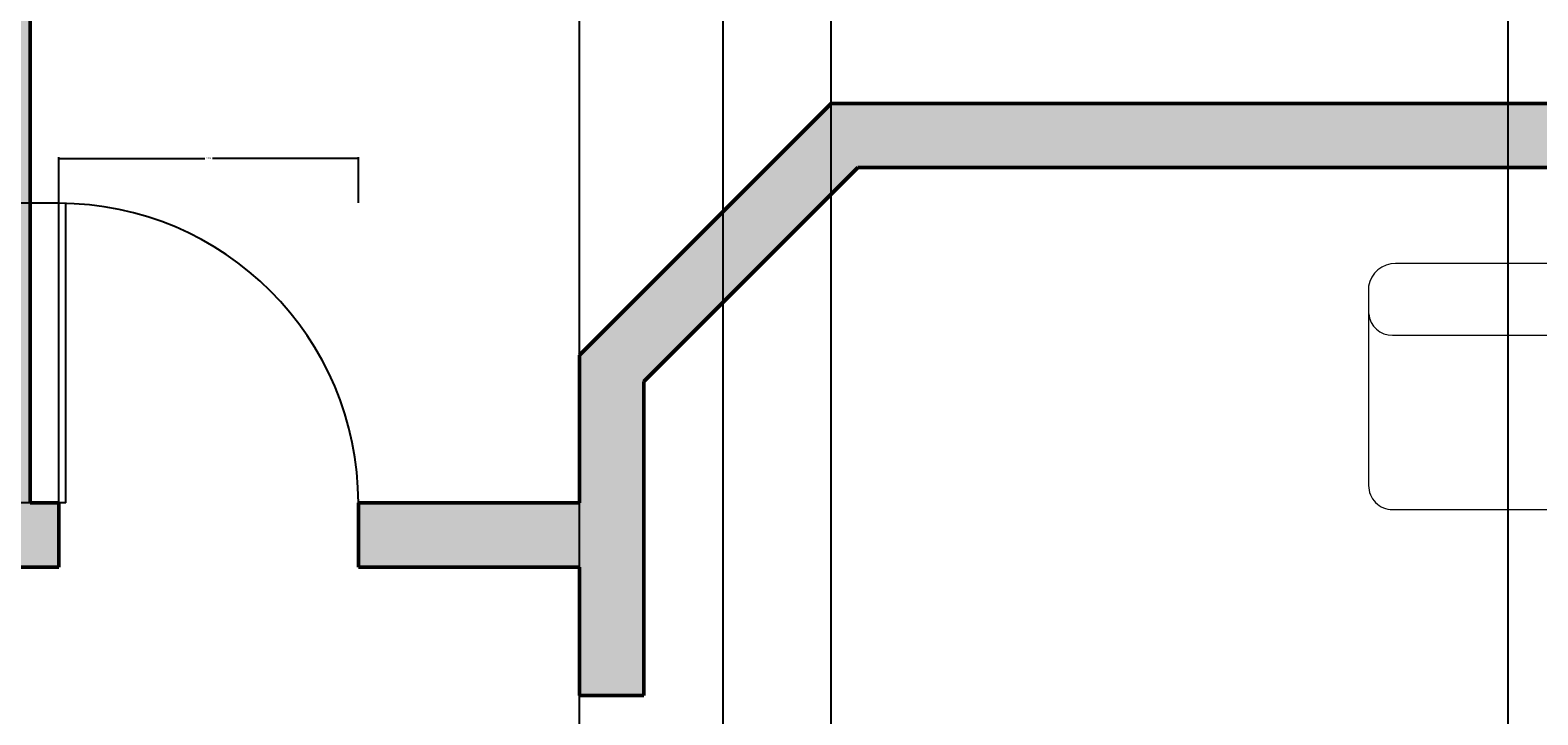
# Model space of a CAD drawing. Units: inches. Extents: x 2447 to 3157, y 2799 to 3988.
# Tile 4 of 9: x 2735 to 2947, y 3345 to 3441. Entities that reach past the tile are written whole.
import ezdxf

# ---------------------------------------------------------------- set-up
doc = ezdxf.new("R2010")
doc.units = ezdxf.units.IN
for name, color, linetype, lineweight in [('A-ANNO-DIMS', 2, 'Continuous', 18), ('A-DOOR', 3, 'Continuous', 25), ('A-FURN', 8, 'Continuous', 18), ('A-WALL', 7, 'Continuous', 50), ('A-WALL-PATT', 252, 'Continuous', 13)]:
    doc.layers.add(name, color=color, linetype=linetype, lineweight=lineweight)
doc.styles.get("Standard").update_dxf_attribs({"font": 'arial.ttf'})
doc.dimstyles.get("Standard").update_dxf_attribs({"dimtxt": 0.18, "dimasz": 0.18, "dimexe": 0.18, "dimexo": 0.0625, "dimgap": 0.09, "dimtad": 0, "dimtih": 1, "dimtoh": 1, "dimdec": 4, "dimzin": 0, "dimdsep": 46, "dimtxsty": 'Standard', "dimcen": 0.09, "dimadec": 0, "dimazin": 0, "dimtfac": 1, "dimtdec": 4, "dimtofl": 0, "dimtmove": 0, "dimatfit": 3, "dimfxl": 1, "dimtolj": 1, "dimtzin": 0, "dimarcsym": 0})

# ---------------------------------------------------------------- blocks, each defined once
blk = doc.blocks.new('A$C2F471D6A')
for p, q in [((2695.9, 2657.3), (2692.2, 1939.9)), ((1797.2, 841.3), (2182.6, 1242.6)), ((1797.2, 833.9), (2189.8, 1242.6)), ((1797.2, 826.4), (2197, 1242.6)), ((1797.2, 818.9), (2204.2, 1242.6)), ((1797.2, 848.8), (2175.4, 1242.6)), ((2161.4, 709.9), (2615.3, 1243.3)), ((2168.6, 709.9), (2622.5, 1243.3)), ((2175.8, 709.9), (2629.7, 1243.3)), ((2183, 709.9), (2636.9, 1243.3)), ((2190.2, 709.9), (2644.1, 1243.3)), ((2197.4, 709.9), (2651.3, 1243.3)), ((2755.3, 709.9), (2980.5, 1000.5)), ((2762.5, 709.9), (2981.1, 992)), ((2769.7, 709.9), (2981.1, 982.7)), ((2776.9, 709.9), (2981.1, 973.4)), ((2784.1, 709.9), (2981.1, 964.1)), ((807.3, 817.6), (89.9, 821.3))]:
    blk.add_line(p, q)
for points in [[(0, 1730, -0.393715), (947.4, 2744.8)], [(946.9, 2744.9, -1), (937.9, 2487, 1)], [(1060.8, 1939.9, 0.132391), (1145.9, 1873.4), (1778.5, 1873.4, 0.326313), (1874.7, 1943.6), (1874.7, 2657.3, 0.389129), (1793.3, 2746), (1149.6, 2746, 0.426582), (1064.5, 2657.3, 0.287811)], [(1060.8, 2545.7, 0.132391), (1145.9, 2479.2), (1778.5, 2479.2, 0.287096), (1869.3, 2536)], [(1878.2, 2536, 0.331063), (1959.6, 2475.5), (2433.2, 2475.5)], [(2433.2, 2475.5), (2592.3, 2475.5, 0.316456), (2692.2, 2545.7, 0.132391), (2777.2, 2479.2), (3409.9, 2479.2, 0.287096), (3500.7, 2536)], [(252.5, 1720.4), (252.5, 1729.1, -0.399385), (979.3, 2493.9)], [(812.9, 1633.4, 0.469502), (1063.7, 1935.5, -1.204519)], [(252.5, 1720.4, -0.77294), (0, 1730, -1)], [(257.4, 558.6), (257.4, 717.7, 0.316456), (187.2, 817.6, 0.132391), (253.7, 902.7), (253.7, 1535.3, 0.326313), (183.5, 1631.5), (180.9, 1631.5, 0.389129)], [(180.9, 0.4, 0.385191), (257.4, 85.1), (257.4, 558.6)]]:
    blk.add_lwpolyline(points, format="xyb")
for points in [[(2433.2, 1869.7), (2592.3, 1869.7, 0.316456), (2692.2, 1939.9, 0.132391), (2777.2, 1873.4), (3409.9, 1873.4, 0.326313), (3506.1, 1943.6), (3506.1, 2657.3, 0.389129), (3424.7, 2746), (2780.9, 2746, 0.426582), (2695.9, 2657.3, 0.287811), (2596, 2746), (1970.7, 2746, 0.366167), (1874.5, 2664.7), (1874.5, 1954.7, 0.414362), (1959.6, 1869.7)], [(877.5, 558.6), (877.5, 717.7, 0.316456), (807.3, 817.6, 0.132391), (873.8, 902.7), (873.8, 1535.3, 0.326313), (803.6, 1631.5), (89.9, 1631.5, 0.389129), (1.2, 1550.1), (1.2, 906.4, 0.426582), (89.9, 821.3, 0.287811), (1.2, 721.4), (1.2, 96.2, 0.366167), (82.5, 0), (792.5, 0, 0.414362), (877.5, 85.1)]]:
    blk.add_lwpolyline(points, format="xyb", close=True)
blk.add_lwpolyline([(1064.5, 2657.3), (1060.8, 1939.9)])
for points in [[(1742.1, 652.3), (1742.1, 1300.3), (3038.1, 1300.3), (3038.1, 652.3)], [(2981.1, 1185.5), (2920, 1185.5), (2920, 1242.6), (1860.2, 1242.6), (1860.2, 1185.5), (1797.2, 1185.5), (1797.2, 762.2), (1860.2, 762.2), (1860.2, 709.1), (2920, 709.1), (2920, 762.2), (2981.1, 762.2)]]:
    blk.add_lwpolyline(points, close=True)
blk = doc.blocks.new('DOOR-SWING-42IN')
for p, q in [((0, 0), (0, 42)), ((1, 0), (1, 41.99)), ((1, 0), (0, 0))]:
    blk.add_line(p, q)
blk.add_arc((0, 0), 42, 0, 90)
blk = doc.blocks.new('*D20')
at = {"layer": 'A-ANNO-DIMS', "color": 0, "lineweight": -2, "transparency": 16777216}
for p, q in [((2739.3, 3416.7), (2732.89, 3416.7)), ((2733.07, 3416.52), (2733.07, 3395.88)), ((2733.07, 3374.88), (2733.07, 3395.52)), ((2739.3, 3374.7), (2732.89, 3374.7))]:
    blk.add_line(p, q, dxfattribs=at)
at = {"layer": 'A-ANNO-DIMS', "color": 0, "transparency": 16777216}
for points in [[(2733.04, 3416.52), (2733.1, 3416.52), (2733.07, 3416.7)], [(2733.04, 3374.88), (2733.1, 3374.88), (2733.07, 3374.7)]]:
    blk.add_solid(points, dxfattribs=at)
at = {"layer": 'Defpoints', "color": 0, "transparency": 16777216}
for p in [(2733.07, 3416.7), (2739.37, 3416.7), (2739.37, 3374.7)]:
    blk.add_point(p, dxfattribs=at)
at = {"layer": 'A-ANNO-DIMS', "color": 0, "transparency": 16777216, "insert": (2733.07, 3395.7), "char_height": 0.18, "attachment_point": 5}
blk.add_mtext('\\A1;DOOR 42 TYP.', dxfattribs=at)
blk = doc.blocks.new('*D21')
at = {"layer": 'A-ANNO-DIMS', "color": 0, "lineweight": -2, "transparency": 16777216}
for p, q in [((2739.37, 3416.76), (2739.37, 3423.18)), ((2781.37, 3416.76), (2781.37, 3423.18)), ((2739.55, 3423), (2759.84, 3423)), ((2781.19, 3423), (2760.9, 3423))]:
    blk.add_line(p, q, dxfattribs=at)
at = {"layer": 'A-ANNO-DIMS', "color": 0, "transparency": 16777216}
for points in [[(2739.55, 3423.03), (2739.55, 3422.97), (2739.37, 3423)], [(2781.19, 3423.03), (2781.19, 3422.97), (2781.37, 3423)]]:
    blk.add_solid(points, dxfattribs=at)
at = {"layer": 'Defpoints', "color": 0, "transparency": 16777216}
for p in [(2781.37, 3423), (2739.37, 3416.7), (2781.37, 3416.7)]:
    blk.add_point(p, dxfattribs=at)
at = {"layer": 'A-ANNO-DIMS', "color": 0, "transparency": 16777216, "insert": (2760.37, 3423), "char_height": 0.18, "attachment_point": 5}
blk.add_mtext('\\A1;42 TYP.', dxfattribs=at)
blk = doc.blocks.new('*D47')
at = {"layer": 'A-ANNO-DIMS', "color": 0, "lineweight": -2, "transparency": 16777216}
for p, q in [((2798.43, 3849.7), (3156.7, 3849.7)), ((3156.52, 3849.52), (3156.52, 3487.38)), ((3156.52, 3124.88), (3156.52, 3487.02)), ((3046.43, 3124.7), (3156.7, 3124.7))]:
    blk.add_line(p, q, dxfattribs=at)
at = {"layer": 'A-ANNO-DIMS', "color": 0, "transparency": 16777216}
for points in [[(3156.49, 3849.52), (3156.55, 3849.52), (3156.52, 3849.7)], [(3156.49, 3124.88), (3156.55, 3124.88), (3156.52, 3124.7)]]:
    blk.add_solid(points, dxfattribs=at)
at = {"layer": 'Defpoints', "color": 0, "transparency": 16777216}
for p in [(2798.37, 3849.7), (3156.52, 3849.7), (3046.37, 3124.7)]:
    blk.add_point(p, dxfattribs=at)
at = {"layer": 'A-ANNO-DIMS', "color": 0, "transparency": 16777216, "insert": (3156.52, 3487.2), "char_height": 0.18, "attachment_point": 5}
blk.add_mtext('\\A1;725', dxfattribs=at)
blk = doc.blocks.new('*D50')
at = {"layer": 'A-ANNO-DIMS', "color": 0, "lineweight": -2, "transparency": 16777216}
for p, q in [((2832.46, 3897.64), (2832.46, 2799.37)), ((2942.46, 3897.64), (2942.46, 2799.37)), ((2832.64, 2799.55), (2887.18, 2799.55)), ((2942.28, 2799.55), (2887.74, 2799.55))]:
    blk.add_line(p, q, dxfattribs=at)
at = {"layer": 'A-ANNO-DIMS', "color": 0, "transparency": 16777216}
for points in [[(2832.64, 2799.58), (2832.64, 2799.52), (2832.46, 2799.55)], [(2942.28, 2799.58), (2942.28, 2799.52), (2942.46, 2799.55)]]:
    blk.add_solid(points, dxfattribs=at)
at = {"layer": 'Defpoints', "color": 0, "transparency": 16777216}
for p in [(2832.46, 3897.7), (2942.46, 3897.7), (2942.46, 2799.55)]:
    blk.add_point(p, dxfattribs=at)
at = {"layer": 'A-ANNO-DIMS', "color": 0, "transparency": 16777216, "insert": (2887.46, 2799.55), "char_height": 0.18, "attachment_point": 5}
blk.add_mtext('\\A1;110', dxfattribs=at)
blk = doc.blocks.new('*D73')
at = {"layer": 'A-ANNO-DIMS', "color": 0, "lineweight": -2, "transparency": 16777216}
for p, q in [((2812.37, 3160.03), (2812.37, 3988.03)), ((2812.55, 3987.85), (2829.61, 3987.85)), ((2847.46, 3987.85), (2830.4, 3987.85)), ((2847.64, 3124.76), (2847.64, 3988.03))]:
    blk.add_line(p, q, dxfattribs=at)
at = {"layer": 'A-ANNO-DIMS', "color": 0, "transparency": 16777216}
for points in [[(2812.55, 3987.88), (2812.55, 3987.82), (2812.37, 3987.85)], [(2847.46, 3987.88), (2847.46, 3987.82), (2847.64, 3987.85)]]:
    blk.add_solid(points, dxfattribs=at)
at = {"layer": 'Defpoints', "color": 0, "transparency": 16777216}
for p in [(2847.64, 3987.85), (2812.37, 3159.97), (2847.64, 3124.7)]:
    blk.add_point(p, dxfattribs=at)
at = {"layer": 'A-ANNO-DIMS', "color": 0, "transparency": 16777216, "insert": (2830, 3987.85), "char_height": 0.18, "attachment_point": 5}
blk.add_mtext('\\A1;35.27', dxfattribs=at)
blk = doc.blocks.new('*D76')
at = {"layer": 'A-ANNO-DIMS', "color": 0, "lineweight": -2, "transparency": 16777216}
for p, q in [((2847.64, 3124.76), (2847.64, 3988.03)), ((2847.82, 3987.85), (2908.95, 3987.85)), ((2970.99, 3987.85), (2909.86, 3987.85)), ((2971.17, 3124.76), (2971.17, 3988.03))]:
    blk.add_line(p, q, dxfattribs=at)
at = {"layer": 'A-ANNO-DIMS', "color": 0, "transparency": 16777216}
for points in [[(2847.82, 3987.88), (2847.82, 3987.82), (2847.64, 3987.85)], [(2970.99, 3987.88), (2970.99, 3987.82), (2971.17, 3987.85)]]:
    blk.add_solid(points, dxfattribs=at)
at = {"layer": 'Defpoints', "color": 0, "transparency": 16777216}
for p in [(2971.17, 3987.85), (2847.64, 3124.7), (2971.17, 3124.7)]:
    blk.add_point(p, dxfattribs=at)
at = {"layer": 'A-ANNO-DIMS', "color": 0, "transparency": 16777216, "insert": (2909.4, 3987.85), "char_height": 0.18, "attachment_point": 5}
blk.add_mtext('\\A1;123.53', dxfattribs=at)

msp = doc.modelspace()

# ---------------------------------------------------------------- hatches: boundary and pattern name
at = {"layer": 'A-WALL-PATT'}
h = msp.add_hatch(color=256, dxfattribs=at)
h.dxf.hatch_style = 1
h.paths.add_polyline_path([(2570.3672, 3550.7002), (2726.3672, 3550.7002), (2726.3672, 3370.7002), (2722.3672, 3370.7002), (2722.3672, 3365.7002), (2739.3672, 3365.7002), (2739.3672, 3374.7002), (2735.3672, 3374.7002), (2735.3672, 3563.7002), (2726.3672, 3563.7002), (2726.3672, 3559.7002), (2570.3672, 3559.7002), (2570.3672, 3599.2479), (2561.3672, 3599.2479), (2561.3672, 3508.7002), (2570.3672, 3508.7002)])
h.paths.add_polyline_path([(2570.3672, 3412.7002), (2561.3672, 3412.7002), (2561.3672, 3331.9279), (2570.3672, 3331.9279), (2570.3672, 3365.7002), (2666.3672, 3365.7002), (2666.3672, 3361.7002), (2671.3672, 3361.7002), (2671.3672, 3365.7002), (2686.3672, 3365.7002), (2686.3672, 3370.7002), (2570.3672, 3370.7002)])
h.paths.add_polyline_path([(2965.3672, 3430.7002), (2961.3672, 3430.7002), (2961.3672, 3434.7002), (2952.3672, 3434.7002), (2952.3672, 3430.7002), (2847.6393, 3430.7002), (2812.3672, 3395.4282), (2812.3672, 3374.7002), (2781.3672, 3374.7002), (2781.3672, 3365.7002), (2812.3672, 3365.7002), (2812.3672, 3347.7002), (2821.3672, 3347.7002), (2821.3672, 3391.7002), (2851.3672, 3421.7002), (2965.3672, 3421.7002)])
h.paths.add_polyline_path([(3046.3672, 3430.7002), (3033.3672, 3430.7002), (3033.3672, 3421.7002), (3037.3672, 3421.7002), (3037.3672, 3133.7002), (2971.1661, 3133.7002), (2971.1661, 3124.7002), (3046.3672, 3124.7002)])
h.paths.add_polyline_path([(3046.3672, 3825.7002), (3005.5801, 3825.7002), (3005.5801, 3816.7002), (3037.3672, 3816.7002), (3037.3672, 3655.7002), (2940.3672, 3655.7002), (2940.3672, 3646.7002), (3037.3672, 3646.7002), (3037.3672, 3514.7002), (3033.3672, 3514.7002), (3033.3672, 3505.7002), (3046.3672, 3505.7002)])
h.paths.add_polyline_path([(2821.3672, 3258.7002), (2812.3672, 3258.7002), (2812.3672, 3240.7002), (2808.3672, 3240.7002), (2808.3672, 3231.7002), (2812.3672, 3231.7002), (2812.3672, 3223.0688), (2821.3672, 3223.0688)])
h.paths.add_polyline_path([(2766.3672, 3240.7002), (2707.3672, 3240.7002), (2707.3672, 3234.4466, -1), (2570.3672, 3234.4466), (2570.3672, 3240.5271), (2561.3672, 3240.5271), (2561.3672, 3234.4466, 0.98243292), (2716.3185, 3231.7002), (2766.3672, 3231.7002)])
h.paths.add_polyline_path([(2570.3672, 3307.9279), (2561.3672, 3307.9279), (2561.3672, 3281.7773), (2570.3672, 3281.7773), (2570.3672, 3284.7002), (2671.3672, 3284.7002), (2671.3672, 3331.7002), (2666.3672, 3331.7002), (2666.3672, 3293.7002), (2570.3672, 3293.7002)])
h.paths.add_polyline_path([(2570.3672, 3739.7002), (2574.3672, 3739.7002), (2574.3672, 3744.7002), (2570.3672, 3744.7002), (2570.3672, 3840.7002), (2614.3672, 3840.7002), (2614.3672, 3849.7002), (2561.3672, 3849.7002), (2561.3672, 3671.2479), (2570.3672, 3671.2479)])
h.paths.add_polyline_path([(2735.3672, 3840.7002), (2789.3672, 3840.7002), (2789.3672, 3816.7002), (2798.3672, 3816.7002), (2798.3672, 3849.7002), (2679.3672, 3849.7002), (2679.3672, 3840.7002), (2726.3672, 3840.7002), (2726.3672, 3778.7002), (2735.3672, 3778.7002)])
h.paths.add_polyline_path([(2651.3672, 3840.7002), (2655.3672, 3840.7002), (2655.3672, 3849.7002), (2638.3672, 3849.7002), (2638.3672, 3840.7002), (2642.3672, 3840.7002), (2642.3672, 3744.7002), (2610.3672, 3744.7002), (2610.3672, 3739.7002), (2726.3672, 3739.7002), (2726.3672, 3599.7002), (2735.3672, 3599.7002), (2735.3672, 3622.7002), (2739.3672, 3622.7002), (2739.3672, 3631.7002), (2735.3672, 3631.7002), (2735.3672, 3748.7002), (2726.3672, 3748.7002), (2726.3672, 3744.7002), (2651.3672, 3744.7002)])
h.paths.add_polyline_path([(2900.3672, 3816.7002), (2904.3672, 3816.7002), (2904.3672, 3825.7002), (2882.3672, 3825.7002), (2882.3672, 3816.7002), (2891.3672, 3816.7002), (2891.3672, 3650.4282), (2872.6393, 3631.7002), (2775.3672, 3631.7002), (2775.3672, 3622.7002), (2876.3672, 3622.7002), (2900.3672, 3646.7002), (2904.3672, 3646.7002), (2904.3672, 3655.7002), (2900.3672, 3655.7002)])
h.paths.add_polyline_path([(2957.5801, 3825.7002), (2940.3672, 3825.7002), (2940.3672, 3816.7002), (2957.5801, 3816.7002)], flags=17)

# ---------------------------------------------------------------- linework, layer by layer
at = {"layer": 'A-WALL'}
for p, q in [((2735.3672, 3563.7002), (2735.3672, 3374.7002)), ((2812.3672, 3395.4282), (2847.6393, 3430.7002)), ((2952.3672, 3430.7002), (2847.6393, 3430.7002)), ((2821.3672, 3391.7002), (2851.3672, 3421.7002)), ((3037.3672, 3421.7002), (2851.3672, 3421.7002)), ((2812.3672, 3395.4282), (2812.3672, 3374.7002)), ((2821.3672, 3391.7002), (2821.3672, 3347.7002)), ((2735.3672, 3374.7002), (2739.3672, 3374.7002)), ((2739.3672, 3374.7002), (2739.3672, 3365.7002)), ((2781.3672, 3374.7002), (2781.3672, 3365.7002)), ((2781.3672, 3374.7002), (2812.3672, 3374.7002)), ((2722.3672, 3365.7002), (2739.3672, 3365.7002)), ((2781.3672, 3365.7002), (2812.3672, 3365.7002)), ((2812.3672, 3365.7002), (2812.3672, 3347.7002)), ((2812.3672, 3347.7002), (2821.3672, 3347.7002))]:
    msp.add_line(p, q, dxfattribs=at)

# ---------------------------------------------------------------- block references
at = {"layer": 'A-DOOR'}
msp.add_blockref('DOOR-SWING-42IN', (2739.3672, 3374.7002), dxfattribs=at)
at = {"layer": 'A-FURN', "xscale": 0.0393700787401575, "yscale": 0.0393700787401575, "zscale": 0.0393700787401575, "rotation": 270}
msp.add_blockref('A$C2F471D6A', (2922.9523, 3408.3287), dxfattribs=at)

# ---------------------------------------------------------------- dimensions: what is measured, and where the dimension line sits
at = {"layer": 'A-ANNO-DIMS'}
for base, p1, p2, override, picture, middle in [((2847.6393, 3987.8502), (2812.3672, 3159.9723), (2847.6393, 3124.7002), {"dimdec": 2, "dimlfac": 1, "dimrnd": 0, "dimzin": 0, "dimdsep": 46, "dimlunit": 2}, '*D73', (2830.0033, 3987.8502)), ((2971.1661, 3987.8502), (2847.6393, 3124.7002), (2971.1661, 3124.7002), {"dimdec": 2, "dimlfac": 1, "dimrnd": 0, "dimzin": 0, "dimdsep": 46, "dimlunit": 2}, '*D76', (2909.4027, 3987.8502)), ((2942.456, 2799.5502), (2832.456, 3897.7002), (2942.456, 3897.7002), {"dimdec": 0, "dimlfac": 1, "dimrnd": 0, "dimzin": 0, "dimdsep": 46, "dimlunit": 2}, '*D50', (2887.456, 2799.5502))]:
    dim = msp.add_linear_dim(base=base, p1=p1, p2=p2, dimstyle='Standard', override=override, dxfattribs=at)
    dim.commit()
    dim.dimension.update_dxf_attribs({"geometry": picture, "text_midpoint": middle})
dim = msp.add_linear_dim(base=(3156.5172, 3849.7002), p1=(3046.3672, 3124.7002), p2=(2798.3672, 3849.7002), angle=90, dimstyle='Standard', override={"dimdec": 0, "dimlfac": 1, "dimrnd": 0, "dimzin": 0, "dimdsep": 46, "dimlunit": 2}, dxfattribs=at)
dim.commit()
dim.dimension.update_dxf_attribs({"geometry": '*D47', "text_midpoint": (3156.5172, 3487.2002)})
dim = msp.add_linear_dim(base=(2781.3672, 3423.0002), p1=(2739.3672, 3416.7002), p2=(2781.3672, 3416.7002), text='<> TYP.', dimstyle='Standard', override={"dimdec": 0, "dimlfac": 1, "dimrnd": 0, "dimzin": 0, "dimdsep": 46, "dimlunit": 2}, dxfattribs=at)
dim.commit()
dim.dimension.update_dxf_attribs({"geometry": '*D21', "text_midpoint": (2760.3672, 3423.0002)})
dim = msp.add_linear_dim(base=(2733.0672, 3416.7002), p1=(2739.3672, 3374.7002), p2=(2739.3672, 3416.7002), angle=90, text='DOOR <> TYP.', dimstyle='Standard', override={"dimdec": 0, "dimlfac": 1, "dimrnd": 0, "dimzin": 0, "dimdsep": 46, "dimlunit": 2}, dxfattribs=at)
dim.commit()
dim.dimension.update_dxf_attribs({"geometry": '*D20', "text_midpoint": (2733.0672, 3395.7002)})

doc.saveas('drawing.dxf')
